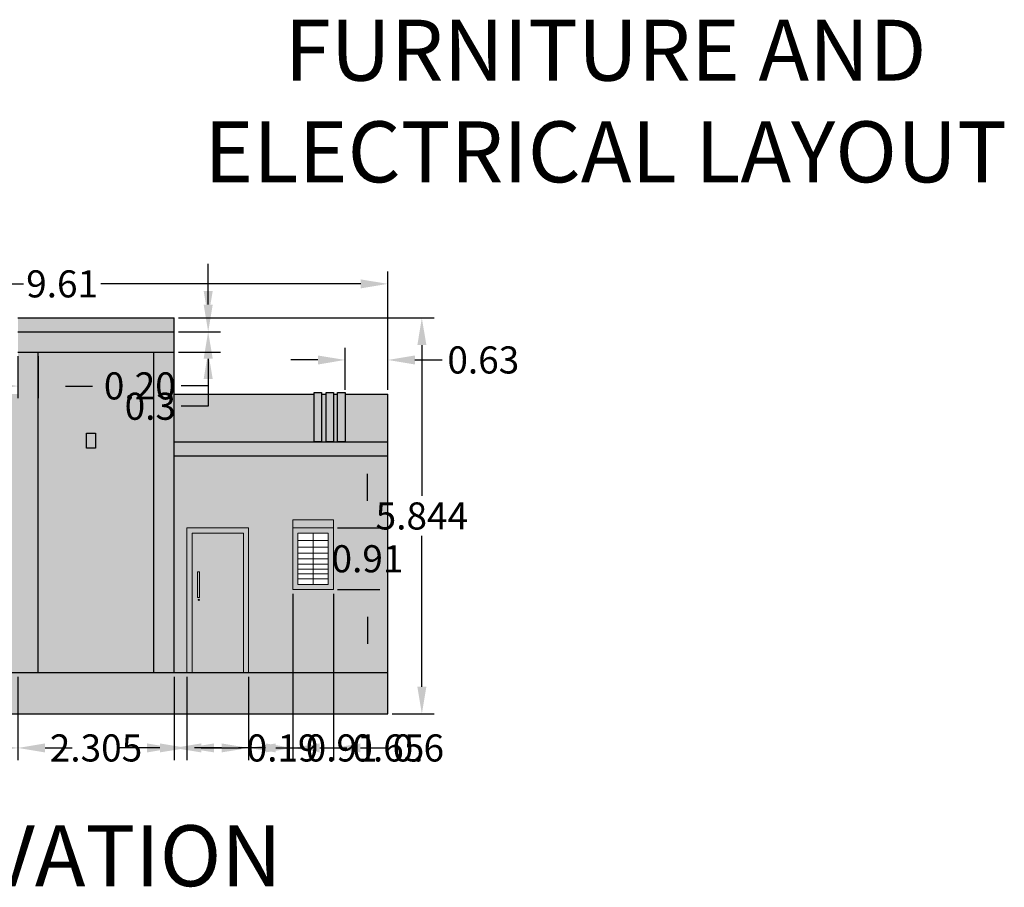
# Model space of a CAD drawing. Units: metres. Extents: x 24.2 to 58.5, y -14.5 to 15.2.
# Tile 3 of 7: x 38.9 to 53.4, y -14.5 to -1.7. Entities that reach past the tile are written whole.
import ezdxf

# ---------------------------------------------------------------- set-up
doc = ezdxf.new("R2010")
doc.units = ezdxf.units.M
doc.header["$MEASUREMENT"] = 0
for name, color, linetype, lineweight in [('A-ANNO-TITL', 1, 'Continuous', 30), ('A-DOOR-PATT', 15, 'Continuous', 13), ('A-ELEV', 7, 'Continuous', 25), ('A-ELEV-PATT', 61, 'Continuous', 13), ('A-GLAZ', 15, 'Continuous', 18), ('DIMENSION', 90, 'Continuous', 18), ('DOOR', 15, 'Continuous', 18)]:
    doc.layers.add(name, color=color, linetype=linetype, lineweight=lineweight)
doc.layers.add('A-ELEV-TRIM-PATT', color=251, linetype='Continuous', lineweight=13, true_color=0x636466)
doc.styles.get("Standard").update_dxf_attribs({"font": 'arial.ttf'})
doc.dimstyles.get("Standard").update_dxf_attribs({"dimtxt": 0.4, "dimasz": 0.4, "dimexe": 0.18, "dimexo": 0.0625, "dimgap": 0.09, "dimtad": 0, "dimtih": 1, "dimtoh": 1, "dimdec": 1, "dimzin": 0, "dimdsep": 46, "dimtxsty": 'Standard', "dimcen": 0.09, "dimadec": 0, "dimazin": 0, "dimtfac": 1, "dimtdec": 1, "dimtofl": 0, "dimtmove": 0, "dimatfit": 3, "dimfxl": 1, "dimtolj": 1, "dimtzin": 0, "dimarcsym": 0})

# ---------------------------------------------------------------- blocks, each defined once
blk = doc.blocks.new('PARAPET-TRIPLE-FIN')
for p, q in [((0.11, 0.707), (0.177, 0.707)), ((0.286, 0.707), (0.345, 0.707))]:
    blk.add_line(p, q)
for points in [[(0, 0.731), (0.11, 0.731), (0.11, 0), (0, 0)], [(0, 0.731), (0.11, 0.731), (0.11, 0), (0, 0)], [(0.177, 0.731), (0.286, 0.731), (0.286, 0), (0.177, 0)], [(0.345, 0.731), (0.455, 0.731), (0.455, 0), (0.345, 0)]]:
    blk.add_lwpolyline(points, close=True)
blk = doc.blocks.new('*D81')
at = {"layer": 'Defpoints', "color": 0, "transparency": 16777216}
for p in [(44.284, -5.562), (34.674, -7.188), (44.284, -7.188)]:
    blk.add_point(p, dxfattribs=at)
at = {"layer": 'DIMENSION', "color": 0, "lineweight": -2, "transparency": 16777216}
for p, q in [((34.674, -7.125), (34.674, -5.382)), ((44.284, -7.125), (44.284, -5.382)), ((35.074, -5.562), (38.908, -5.562)), ((43.884, -5.562), (40.05, -5.562))]:
    blk.add_line(p, q, dxfattribs=at)
at = {"layer": 'DIMENSION', "color": 0, "transparency": 16777216}
for points in [[(35.074, -5.496), (35.074, -5.629), (34.674, -5.562)], [(43.884, -5.496), (43.884, -5.629), (44.284, -5.562)]]:
    blk.add_solid(points, dxfattribs=at)
at = {"layer": 'DIMENSION', "color": 0, "transparency": 16777216, "insert": (39.479, -5.562), "char_height": 0.4, "attachment_point": 5}
blk.add_mtext('\\A1;9.61', dxfattribs=at)
blk = doc.blocks.new('*D82')
at = {"layer": 'Defpoints', "color": 0, "transparency": 16777216}
for p in [(41.131, -6.065), (44.786, -6.065), (44.284, -11.908)]:
    blk.add_point(p, dxfattribs=at)
at = {"layer": 'DIMENSION', "color": 0, "lineweight": -2, "transparency": 16777216}
for p, q in [((41.194, -6.065), (44.966, -6.065)), ((44.786, -6.465), (44.786, -8.692)), ((44.786, -11.508), (44.786, -9.281)), ((44.346, -11.908), (44.966, -11.908))]:
    blk.add_line(p, q, dxfattribs=at)
at = {"layer": 'DIMENSION', "color": 0, "transparency": 16777216}
for points in [[(44.72, -6.465), (44.853, -6.465), (44.786, -6.065)], [(44.72, -11.508), (44.853, -11.508), (44.786, -11.908)]]:
    blk.add_solid(points, dxfattribs=at)
at = {"layer": 'DIMENSION', "color": 0, "transparency": 16777216, "insert": (44.786, -8.987), "char_height": 0.4, "attachment_point": 5}
blk.add_mtext('\\A1;5.844', dxfattribs=at)
blk = doc.blocks.new('*D89')
at = {"layer": 'Defpoints', "color": 0, "transparency": 16777216}
for p in [(43.481, -9.164), (43.481, -10.074), (43.984, -10.074)]:
    blk.add_point(p, dxfattribs=at)
at = {"layer": 'DIMENSION', "color": 0, "lineweight": -2, "transparency": 16777216}
for p, q in [((43.984, -8.764), (43.984, -8.364)), ((43.544, -9.164), (44.164, -9.164)), ((43.544, -10.074), (44.164, -10.074)), ((43.984, -10.474), (43.984, -10.874))]:
    blk.add_line(p, q, dxfattribs=at)
at = {"layer": 'DIMENSION', "color": 0, "transparency": 16777216}
for points in [[(43.917, -8.764), (44.05, -8.764), (43.984, -9.164)], [(43.917, -10.474), (44.05, -10.474), (43.984, -10.074)]]:
    blk.add_solid(points, dxfattribs=at)
at = {"layer": 'DIMENSION', "color": 0, "transparency": 16777216, "insert": (43.984, -9.619), "char_height": 0.4, "attachment_point": 5}
blk.add_mtext('\\A1;0.91', dxfattribs=at)
blk = doc.blocks.new('*D92')
at = {"layer": 'Defpoints', "color": 0, "transparency": 16777216}
for p in [(37.437, -10.388), (38.827, -11.298), (38.827, -12.411)]:
    blk.add_point(p, dxfattribs=at)
at = {"layer": 'DIMENSION', "color": 0, "lineweight": -2, "transparency": 16777216}
for p, q in [((37.437, -10.451), (37.437, -12.591)), ((38.827, -11.361), (38.827, -12.591)), ((37.037, -12.411), (36.637, -12.411)), ((39.227, -12.411), (39.627, -12.411))]:
    blk.add_line(p, q, dxfattribs=at)
at = {"layer": 'DIMENSION', "color": 0, "transparency": 16777216}
for points in [[(37.037, -12.344), (37.037, -12.477), (37.437, -12.411)], [(39.227, -12.344), (39.227, -12.477), (38.827, -12.411)]]:
    blk.add_solid(points, dxfattribs=at)
at = {"layer": 'DIMENSION', "color": 0, "transparency": 16777216, "insert": (38.132, -12.411), "char_height": 0.4, "attachment_point": 5}
blk.add_mtext('\\A1;1.39', dxfattribs=at)
blk = doc.blocks.new('*D93')
at = {"layer": 'Defpoints', "color": 0, "transparency": 16777216}
for p in [(38.827, -11.298), (41.131, -11.298), (41.131, -12.411)]:
    blk.add_point(p, dxfattribs=at)
at = {"layer": 'DIMENSION', "color": 0, "lineweight": -2, "transparency": 16777216}
for p, q in [((38.827, -11.361), (38.827, -12.591)), ((41.131, -11.361), (41.131, -12.591)), ((38.427, -12.411), (38.027, -12.411)), ((41.531, -12.411), (41.931, -12.411))]:
    blk.add_line(p, q, dxfattribs=at)
at = {"layer": 'DIMENSION', "color": 0, "transparency": 16777216}
for points in [[(38.427, -12.344), (38.427, -12.477), (38.827, -12.411)], [(41.531, -12.344), (41.531, -12.477), (41.131, -12.411)]]:
    blk.add_solid(points, dxfattribs=at)
at = {"layer": 'DIMENSION', "color": 0, "transparency": 16777216, "insert": (39.979, -12.411), "char_height": 0.4, "attachment_point": 5}
blk.add_mtext('\\A1;2.305', dxfattribs=at)
blk = doc.blocks.new('*D94')
at = {"layer": 'Defpoints', "color": 0, "transparency": 16777216}
for p in [(41.131, -11.298), (41.321, -11.298), (41.321, -12.411)]:
    blk.add_point(p, dxfattribs=at)
at = {"layer": 'DIMENSION', "color": 0, "lineweight": -2, "transparency": 16777216}
for p, q in [((41.131, -11.361), (41.131, -12.591)), ((41.321, -11.361), (41.321, -12.591)), ((40.731, -12.411), (40.331, -12.411)), ((41.721, -12.411), (42.121, -12.411))]:
    blk.add_line(p, q, dxfattribs=at)
at = {"layer": 'DIMENSION', "color": 0, "transparency": 16777216}
for points in [[(40.731, -12.344), (40.731, -12.477), (41.131, -12.411)], [(41.721, -12.344), (41.721, -12.477), (41.321, -12.411)]]:
    blk.add_solid(points, dxfattribs=at)
at = {"layer": 'DIMENSION', "color": 0, "transparency": 16777216, "insert": (42.731, -12.411), "char_height": 0.4, "attachment_point": 5}
blk.add_mtext('\\A1;0.19', dxfattribs=at)
blk = doc.blocks.new('*D95')
at = {"layer": 'Defpoints', "color": 0, "transparency": 16777216}
for p in [(41.321, -11.298), (42.231, -11.298), (42.231, -12.411)]:
    blk.add_point(p, dxfattribs=at)
at = {"layer": 'DIMENSION', "color": 0, "lineweight": -2, "transparency": 16777216}
for p, q in [((41.321, -11.361), (41.321, -12.591)), ((42.231, -11.361), (42.231, -12.591)), ((40.921, -12.411), (40.521, -12.411)), ((42.631, -12.411), (43.031, -12.411))]:
    blk.add_line(p, q, dxfattribs=at)
at = {"layer": 'DIMENSION', "color": 0, "transparency": 16777216}
for points in [[(40.921, -12.344), (40.921, -12.477), (41.321, -12.411)], [(42.631, -12.344), (42.631, -12.477), (42.231, -12.411)]]:
    blk.add_solid(points, dxfattribs=at)
at = {"layer": 'DIMENSION', "color": 0, "transparency": 16777216, "insert": (43.602, -12.411), "char_height": 0.4, "attachment_point": 5}
blk.add_mtext('\\A1;0.91', dxfattribs=at)
blk = doc.blocks.new('*D96')
at = {"layer": 'Defpoints', "color": 0, "transparency": 16777216}
for p in [(42.881, -10.074), (42.231, -11.298), (42.881, -12.411)]:
    blk.add_point(p, dxfattribs=at)
at = {"layer": 'DIMENSION', "color": 0, "lineweight": -2, "transparency": 16777216}
for p, q in [((42.881, -10.137), (42.881, -12.591)), ((42.231, -11.361), (42.231, -12.591)), ((41.831, -12.411), (41.431, -12.411)), ((43.281, -12.411), (43.681, -12.411))]:
    blk.add_line(p, q, dxfattribs=at)
at = {"layer": 'DIMENSION', "color": 0, "transparency": 16777216}
for points in [[(41.831, -12.344), (41.831, -12.477), (42.231, -12.411)], [(43.281, -12.344), (43.281, -12.477), (42.881, -12.411)]]:
    blk.add_solid(points, dxfattribs=at)
at = {"layer": 'DIMENSION', "color": 0, "transparency": 16777216, "insert": (44.292, -12.411), "char_height": 0.4, "attachment_point": 5}
blk.add_mtext('\\A1;0.65', dxfattribs=at)
blk = doc.blocks.new('*D97')
at = {"layer": 'Defpoints', "color": 0, "transparency": 16777216}
for p in [(42.881, -10.074), (43.481, -10.074), (43.481, -12.411)]:
    blk.add_point(p, dxfattribs=at)
at = {"layer": 'DIMENSION', "color": 0, "lineweight": -2, "transparency": 16777216}
for p, q in [((42.881, -10.137), (42.881, -12.591)), ((43.481, -10.137), (43.481, -12.591)), ((42.481, -12.411), (42.081, -12.411)), ((43.881, -12.411), (44.281, -12.411))]:
    blk.add_line(p, q, dxfattribs=at)
at = {"layer": 'DIMENSION', "color": 0, "transparency": 16777216}
for points in [[(42.481, -12.344), (42.481, -12.477), (42.881, -12.411)], [(43.881, -12.344), (43.881, -12.477), (43.481, -12.411)]]:
    blk.add_solid(points, dxfattribs=at)
at = {"layer": 'DIMENSION', "color": 0, "transparency": 16777216, "insert": (44.735, -12.411), "char_height": 0.4, "attachment_point": 5}
blk.add_mtext('\\A1;0.6', dxfattribs=at)
blk = doc.blocks.new('*D99')
at = {"layer": 'Defpoints', "color": 0, "transparency": 16777216}
for p in [(44.284, -6.685), (43.653, -7.188), (44.284, -7.188)]:
    blk.add_point(p, dxfattribs=at)
at = {"layer": 'DIMENSION', "color": 0, "lineweight": -2, "transparency": 16777216}
for p, q in [((43.653, -7.125), (43.653, -6.505)), ((44.284, -7.125), (44.284, -6.505)), ((43.253, -6.685), (42.853, -6.685)), ((44.684, -6.685), (45.084, -6.685))]:
    blk.add_line(p, q, dxfattribs=at)
at = {"layer": 'DIMENSION', "color": 0, "transparency": 16777216}
for points in [[(43.253, -6.619), (43.253, -6.752), (43.653, -6.685)], [(44.684, -6.619), (44.684, -6.752), (44.284, -6.685)]]:
    blk.add_solid(points, dxfattribs=at)
at = {"layer": 'DIMENSION', "color": 0, "transparency": 16777216, "insert": (45.693, -6.685), "char_height": 0.4, "attachment_point": 5}
blk.add_mtext('\\A1;0.63', dxfattribs=at)
blk = doc.blocks.new('*D100')
at = {"layer": 'Defpoints', "color": 0, "transparency": 16777216}
for p in [(41.131, -6.065), (41.131, -6.268), (41.634, -6.268)]:
    blk.add_point(p, dxfattribs=at)
at = {"layer": 'DIMENSION', "color": 0, "lineweight": -2, "transparency": 16777216}
for p, q in [((41.634, -5.665), (41.634, -5.265)), ((41.194, -6.065), (41.814, -6.065)), ((41.194, -6.268), (41.814, -6.268)), ((41.634, -6.668), (41.634, -7.068)), ((41.634, -7.068), (41.234, -7.068))]:
    blk.add_line(p, q, dxfattribs=at)
at = {"layer": 'DIMENSION', "color": 0, "transparency": 16777216}
for points in [[(41.567, -5.665), (41.701, -5.665), (41.634, -6.065)], [(41.567, -6.668), (41.701, -6.668), (41.634, -6.268)]]:
    blk.add_solid(points, dxfattribs=at)
at = {"layer": 'DIMENSION', "color": 0, "transparency": 16777216, "insert": (40.625, -7.068), "char_height": 0.4, "attachment_point": 5}
blk.add_mtext('\\A1;0.20', dxfattribs=at)
blk = doc.blocks.new('*D101')
at = {"layer": 'Defpoints', "color": 0, "transparency": 16777216}
for p in [(41.131, -6.268), (41.131, -6.568), (41.634, -6.568)]:
    blk.add_point(p, dxfattribs=at)
at = {"layer": 'DIMENSION', "color": 0, "lineweight": -2, "transparency": 16777216}
for p, q in [((41.634, -5.868), (41.634, -5.468)), ((41.194, -6.268), (41.814, -6.268)), ((41.194, -6.568), (41.814, -6.568)), ((41.634, -6.968), (41.634, -7.368)), ((41.634, -7.368), (41.234, -7.368))]:
    blk.add_line(p, q, dxfattribs=at)
at = {"layer": 'DIMENSION', "color": 0, "transparency": 16777216}
for points in [[(41.567, -5.868), (41.701, -5.868), (41.634, -6.268)], [(41.567, -6.968), (41.701, -6.968), (41.634, -6.568)]]:
    blk.add_solid(points, dxfattribs=at)
at = {"layer": 'DIMENSION', "color": 0, "transparency": 16777216, "insert": (40.78, -7.368), "char_height": 0.4, "attachment_point": 5}
blk.add_mtext('\\A1;0.3', dxfattribs=at)
blk = doc.blocks.new('*D102')
at = {"layer": 'Defpoints', "color": 0, "transparency": 16777216}
for p in [(38.827, -6.568), (39.127, -6.568), (38.827, -7.07)]:
    blk.add_point(p, dxfattribs=at)
at = {"layer": 'DIMENSION', "color": 0, "lineweight": -2, "transparency": 16777216}
for p, q in [((38.827, -6.63), (38.827, -7.25)), ((39.127, -6.63), (39.127, -7.25)), ((38.427, -7.07), (38.027, -7.07)), ((39.527, -7.07), (39.927, -7.07))]:
    blk.add_line(p, q, dxfattribs=at)
at = {"layer": 'DIMENSION', "color": 0, "transparency": 16777216}
for points in [[(38.427, -7.004), (38.427, -7.137), (38.827, -7.07)], [(39.527, -7.004), (39.527, -7.137), (39.127, -7.07)]]:
    blk.add_solid(points, dxfattribs=at)
at = {"layer": 'DIMENSION', "color": 0, "transparency": 16777216, "insert": (37.572, -7.07), "char_height": 0.4, "attachment_point": 5}
blk.add_mtext('\\A1;0.3', dxfattribs=at)

msp = doc.modelspace()

# ---------------------------------------------------------------- hatches: boundary and pattern name
at = {"layer": 'A-DOOR-PATT', "transparency": 33554567}
h = msp.add_hatch(color=256, dxfattribs=at)
h.dxf.hatch_style = 1
h.paths.add_polyline_path([(41.3971, -9.2405), (42.1547, -9.2405), (42.1547, -11.2983), (42.2309, -11.2983), (42.2309, -9.1643), (41.3209, -9.1643), (41.3209, -11.2983), (41.3971, -11.2983)])
h = msp.add_hatch(color=256, dxfattribs=at)
h.dxf.hatch_style = 1
h.paths.add_polyline_path([(41.3971, -11.2983), (42.1547, -11.2983), (42.1547, -9.2405), (41.3971, -9.2405)])
h.paths.add_polyline_path([(41.5043, -10.1885), (41.4776, -10.1885), (41.4776, -9.8121), (41.5043, -9.8121)], flags=16)
at = {"layer": 'A-ELEV-PATT', "transparency": 33554567}
h = msp.add_hatch(color=256, dxfattribs=at)
h.dxf.hatch_style = 1
h.paths.add_polyline_path([(38.8266, -8.0979), (34.6742, -8.0979), (34.6742, -11.2983), (38.8266, -11.2983)])
h.paths.add_polyline_path([(37.4366, -10.3883), (36.2166, -10.3883), (36.2166, -9.1683), (36.2166, -9.0299), (37.4366, -9.0299), (37.4366, -9.1683)], flags=16)
h.paths.add_polyline_path([(37.3604, -10.3121), (36.2928, -10.3121), (36.2928, -9.2445), (36.8012, -9.2445), (37.3604, -9.2445)], flags=0)
h.paths.add_polyline_path([(37.1162, -10.0461), (36.852, -10.0461), (36.852, -9.2445), (37.1162, -9.2445)], flags=0)
h.paths.add_polyline_path([(36.8012, -10.0461), (36.557, -10.0461), (36.557, -9.4996), (36.8012, -9.4996)], flags=0)
h.paths.add_polyline_path([(44.2838, -8.0979), (41.1314, -8.0979), (41.1314, -11.2983), (41.3209, -11.2983), (41.3209, -9.1643), (42.2309, -9.1643), (42.2309, -11.2983), (44.2838, -11.2983)])
h.paths.add_polyline_path([(42.8811, -9.0437), (43.4811, -9.0437), (43.4811, -9.1643), (43.4811, -10.0743), (42.8811, -10.0743), (42.8811, -9.1643)], flags=16)
h.paths.add_polyline_path([(42.9573, -9.2405), (43.4049, -9.2405), (43.4049, -9.9981), (42.9573, -9.9981)], flags=0)
h.paths.add_polyline_path([(44.2838, -7.8947), (41.1314, -7.8947), (41.1314, -8.0979), (44.2838, -8.0979)])
h.paths.add_polyline_path([(38.8266, -7.8947), (34.6742, -7.8947), (34.6742, -8.0979), (38.8266, -8.0979)])
h.paths.add_polyline_path([(41.1314, -6.2679), (38.8266, -6.2679), (38.8266, -6.5679), (41.1314, -6.5679)])
h.paths.add_polyline_path([(39.1266, -6.5679), (38.8266, -6.5679), (38.8266, -11.2983), (39.1266, -11.2983)])
h.paths.add_polyline_path([(41.1314, -6.5679), (40.8314, -6.5679), (40.8314, -11.2983), (41.1314, -11.2983), (41.1314, -8.0979)])
h.paths.add_polyline_path([(35.4837, -7.1642), (35.3742, -7.1642), (35.3742, -7.8947), (35.4837, -7.8947)])
h.paths.add_polyline_path([(35.6603, -7.1642), (35.5509, -7.1642), (35.5509, -7.8947), (35.6603, -7.8947)])
h.paths.add_polyline_path([(35.8286, -7.1642), (35.7192, -7.1642), (35.7192, -7.8947), (35.8286, -7.8947)])
h.paths.add_polyline_path([(43.3078, -7.1642), (43.1983, -7.1642), (43.1983, -7.8947), (43.3078, -7.8947)])
h.paths.add_polyline_path([(43.4844, -7.1642), (43.3749, -7.1642), (43.3749, -7.8947), (43.4844, -7.8947)])
h.paths.add_polyline_path([(43.6527, -7.1642), (43.5433, -7.1642), (43.5433, -7.8947), (43.6527, -7.8947)])
at = {"layer": 'A-ELEV-TRIM-PATT', "transparency": 33554567}
h = msp.add_hatch(color=256, dxfattribs=at)
h.dxf.hatch_style = 1
h.paths.add_polyline_path([(40.8314, -6.5679), (39.1266, -6.5679), (39.1266, -11.2983), (40.8314, -11.2983)])
h.paths.add_polyline_path([(44.2838, -11.2983), (34.6742, -11.2983), (34.6742, -11.9083), (44.2838, -11.9083)])
h.paths.add_polyline_path([(38.8266, -7.1879), (35.8286, -7.1879), (35.8286, -7.8947), (38.8266, -7.8947)])
h.paths.add_polyline_path([(35.3742, -7.1879), (34.6742, -7.1879), (34.6742, -7.8947), (35.3742, -7.8947)])
h.paths.add_polyline_path([(35.5509, -7.1879), (35.4837, -7.1879), (35.4837, -7.8947), (35.5509, -7.8947)])
h.paths.add_polyline_path([(35.7192, -7.1879), (35.6603, -7.1879), (35.6603, -7.8947), (35.7192, -7.8947)])
h.paths.add_polyline_path([(43.1983, -7.1879), (41.1314, -7.1879), (41.1314, -7.8947), (43.1983, -7.8947)])
h.paths.add_polyline_path([(44.2838, -7.1879), (43.6527, -7.1879), (43.6527, -7.8947), (44.2838, -7.8947)])
h.paths.add_polyline_path([(43.3749, -7.1879), (43.3078, -7.1879), (43.3078, -7.8947), (43.3749, -7.8947)])
h.paths.add_polyline_path([(43.5433, -7.1879), (43.4844, -7.1879), (43.4844, -7.8947), (43.5433, -7.8947)])
h.paths.add_polyline_path([(41.1314, -6.0647), (38.8266, -6.0647), (38.8266, -6.2679), (41.1314, -6.2679)])
h = msp.add_hatch(color=256, dxfattribs=at)
h.dxf.hatch_style = 1
h.paths.add_polyline_path([(39.8379, -7.9868), (39.971, -7.9868), (39.971, -7.7651), (39.8379, -7.7651)])
h = msp.add_hatch(color=256, dxfattribs=at)
h.dxf.hatch_style = 1
h.paths.add_polyline_path([(37.4366, -9.1683), (37.4366, -9.0299), (36.2166, -9.0299), (36.2166, -9.1683)])
h.paths.add_polyline_path([(42.8811, -9.0437), (42.8811, -9.1643), (43.4811, -9.1643), (43.4811, -9.0437)])
h = msp.add_hatch(color=256, dxfattribs=at)
h.dxf.hatch_style = 1
h.paths.add_polyline_path([(36.2166, -10.3883), (37.4366, -10.3883), (37.4366, -9.1683), (36.2166, -9.1683)])
h.paths.add_polyline_path([(36.2928, -9.2445), (37.3604, -9.2445), (37.3604, -10.3121), (36.2928, -10.3121)], flags=16)
h.paths.add_polyline_path([(43.4811, -9.1643), (42.8811, -9.1643), (42.8811, -10.0743), (43.4811, -10.0743)])
h.paths.add_polyline_path([(43.4049, -9.9981), (42.9573, -9.9981), (42.9573, -9.2405), (43.4049, -9.2405)], flags=16)
h = msp.add_hatch(color=256, dxfattribs=at)
h.dxf.hatch_style = 1
h.paths.add_polyline_path([(41.5043, -9.8121), (41.4776, -9.8121), (41.4776, -10.1885), (41.5043, -10.1885)])
h.paths.add_polyline_path([(41.4845, -10.2255, 1), (41.504, -10.2255, 1)])

# ---------------------------------------------------------------- linework, layer by layer
at = {"layer": 'A-ELEV'}
for p, q in [((38.8266, -6.0647), (41.1314, -6.0647)), ((41.1314, -11.2983), (41.1314, -6.0647)), ((38.8266, -6.2679), (41.1314, -6.2679)), ((38.8266, -6.5679), (41.1314, -6.5679)), ((39.1266, -11.2983), (39.1266, -6.5679)), ((40.8314, -11.2983), (40.8314, -6.5679)), ((41.1314, -7.1879), (43.1983, -7.1879)), ((43.6527, -7.1879), (44.2838, -7.1879)), ((44.2838, -11.9083), (44.2838, -7.1879)), ((41.1314, -7.8947), (44.2838, -7.8947)), ((41.1314, -8.0979), (44.2838, -8.0979)), ((34.6742, -11.2983), (44.2838, -11.2983)), ((34.6742, -11.9083), (44.2838, -11.9083))]:
    msp.add_line(p, q, dxfattribs=at)
msp.add_lwpolyline([(39.8379, -7.7651), (39.971, -7.7651), (39.971, -7.9868), (39.8379, -7.9868)], close=True, dxfattribs=at)
at = {"layer": 'A-GLAZ'}
for p, q in [((42.8811, -10.0743), (42.8811, -9.1643)), ((42.8811, -9.1643), (43.4811, -9.1643)), ((42.9573, -9.9981), (42.9573, -9.2405)), ((42.9573, -9.2405), (43.4049, -9.2405)), ((43.1811, -9.9981), (43.1811, -9.2405)), ((43.4049, -9.2405), (43.4049, -9.9981)), ((43.4811, -9.1643), (43.4811, -10.0743)), ((42.9573, -9.3504), (43.4049, -9.3504)), ((42.9573, -9.4462), (43.4049, -9.4462)), ((42.9573, -9.5359), (43.4049, -9.5359)), ((42.9573, -9.6193), (43.4049, -9.6193)), ((42.9573, -9.6969), (43.4049, -9.6969)), ((42.9573, -9.7744), (43.4049, -9.7744)), ((42.9573, -9.8437), (43.4049, -9.8437)), ((42.9573, -9.9171), (43.4049, -9.9171)), ((43.4049, -9.9981), (42.9573, -9.9981)), ((43.4811, -10.0743), (42.8811, -10.0743))]:
    msp.add_line(p, q, dxfattribs=at)
msp.add_lwpolyline([(42.8811, -9.1643), (43.4811, -9.1643), (43.4811, -9.0437), (42.8811, -9.0437)], close=True, dxfattribs=at)
at = {"layer": 'DOOR'}
for p, q in [((41.3209, -11.2983), (41.3209, -9.1643)), ((41.3209, -9.1643), (42.2309, -9.1643)), ((41.3971, -11.2983), (41.3971, -9.2405)), ((41.3971, -9.2405), (42.1547, -9.2405)), ((42.1547, -9.2405), (42.1547, -11.2983)), ((42.2309, -9.1643), (42.2309, -11.2983))]:
    msp.add_line(p, q, dxfattribs=at)
msp.add_lwpolyline([(41.4776, -9.8121), (41.5043, -9.8121), (41.5043, -10.1885), (41.4776, -10.1885)], close=True, dxfattribs=at)
msp.add_circle((41.4942, -10.2255), 0.00978, dxfattribs=at)

# ---------------------------------------------------------------- block references
at = {"layer": 'A-ELEV'}
msp.add_blockref('PARAPET-TRIPLE-FIN', (43.1981, -7.895), dxfattribs=at)

# ---------------------------------------------------------------- texts
at = {"layer": 'A-ANNO-TITL', "char_height": 0.9, "attachment_point": 2}
for s, width, insert in [('FURNITURE AND ELECTRICAL LAYOUT', 15.147471, (47.4972, -1.6633)), ('ELEVATION', 1.744906, (39.4872, -13.5517))]:
    msp.add_mtext_dynamic_manual_height_columns(s, width=width, gutter_width=1, heights=[0], dxfattribs=dict(at, insert=insert))

# ---------------------------------------------------------------- dimensions: what is measured, and where the dimension line sits
at = {"layer": 'DIMENSION'}
for base, p1, p2, override, picture, middle in [((44.2838, -5.5622), (34.6742, -7.1879), (44.2838, -7.1879), {"dimdec": 2, "dimlfac": 1, "dimrnd": 0, "dimzin": 0, "dimdsep": 46, "dimlunit": 2}, '*D81', (39.479, -5.5622)), ((44.2838, -6.6854), (43.6527, -7.1879), (44.2838, -7.1879), {"dimdec": 2, "dimlfac": 1, "dimrnd": 0, "dimzin": 0, "dimdsep": 46, "dimlunit": 2}, '*D99', (45.6933, -6.6854)), ((42.8811, -12.4108), (42.2309, -11.2983), (42.8811, -10.0743), {"dimdec": 2, "dimlfac": 1, "dimrnd": 0, "dimzin": 0, "dimdsep": 46, "dimlunit": 2}, '*D96', (44.2921, -12.4108)), ((43.4811, -12.4108), (42.8811, -10.0743), (43.4811, -10.0743), {"dimdec": 1, "dimlfac": 1, "dimrnd": 0, "dimzin": 0, "dimdsep": 46, "dimlunit": 2}, '*D97', (44.7351, -12.4108)), ((38.8266, -12.4108), (37.4366, -10.3883), (38.8266, -11.2983), {"dimdec": 2, "dimlfac": 1, "dimrnd": 0, "dimzin": 0, "dimdsep": 46, "dimlunit": 2}, '*D92', (38.1316, -12.4108)), ((41.1314, -12.4108), (38.8266, -11.2983), (41.1314, -11.2983), {"dimdec": 3, "dimlfac": 1, "dimrnd": 0, "dimzin": 0, "dimdsep": 46, "dimlunit": 2}, '*D93', (39.979, -12.4108)), ((41.3209, -12.4108), (41.1314, -11.2983), (41.3209, -11.2983), {"dimdec": 2, "dimlfac": 1, "dimrnd": 0, "dimzin": 0, "dimdsep": 46, "dimlunit": 2}, '*D94', (42.7308, -12.4108)), ((42.2309, -12.4108), (41.3209, -11.2983), (42.2309, -11.2983), {"dimdec": 2, "dimlfac": 1, "dimrnd": 0, "dimzin": 0, "dimdsep": 46, "dimlunit": 2}, '*D95', (43.6018, -12.4108))]:
    dim = msp.add_linear_dim(base=base, p1=p1, p2=p2, dimstyle='Standard', override=override, dxfattribs=at)
    dim.commit()
    dim.dimension.update_dxf_attribs({"geometry": picture, "text_midpoint": middle})
for base, p1, p2, angle, override, picture, middle in [((41.6339, -6.2679), (41.1314, -6.0647), (41.1314, -6.2679), 270, {"dimdec": 2, "dimlfac": 1, "dimrnd": 0, "dimzin": 0, "dimdsep": 46, "dimlunit": 2}, '*D100', (40.6251, -7.0679)), ((41.6339, -6.5679), (41.1314, -6.2679), (41.1314, -6.5679), 270, {"dimdec": 1, "dimlfac": 1, "dimrnd": 0, "dimzin": 0, "dimdsep": 46, "dimlunit": 2}, '*D101', (40.7798, -7.3679)), ((44.7863, -6.0647), (44.2838, -11.9083), (41.1314, -6.0647), 90, {"dimdec": 3, "dimlfac": 1, "dimrnd": 0, "dimzin": 0, "dimdsep": 46, "dimlunit": 2}, '*D82', (44.7863, -8.9865)), ((38.8266, -7.0704), (39.1266, -6.5679), (38.8266, -6.5679), 180, {"dimdec": 1, "dimlfac": 1, "dimrnd": 0, "dimzin": 0, "dimdsep": 46, "dimlunit": 2}, '*D102', (37.5725, -7.0704)), ((43.9836, -10.0743), (43.4811, -9.1643), (43.4811, -10.0743), 270, {"dimdec": 2, "dimlfac": 1, "dimrnd": 0, "dimzin": 0, "dimdsep": 46, "dimlunit": 2}, '*D89', (43.9836, -9.6193))]:
    dim = msp.add_linear_dim(base=base, p1=p1, p2=p2, angle=angle, dimstyle='Standard', override=override, dxfattribs=at)
    dim.commit()
    dim.dimension.update_dxf_attribs({"geometry": picture, "text_midpoint": middle})

doc.saveas('drawing.dxf')
